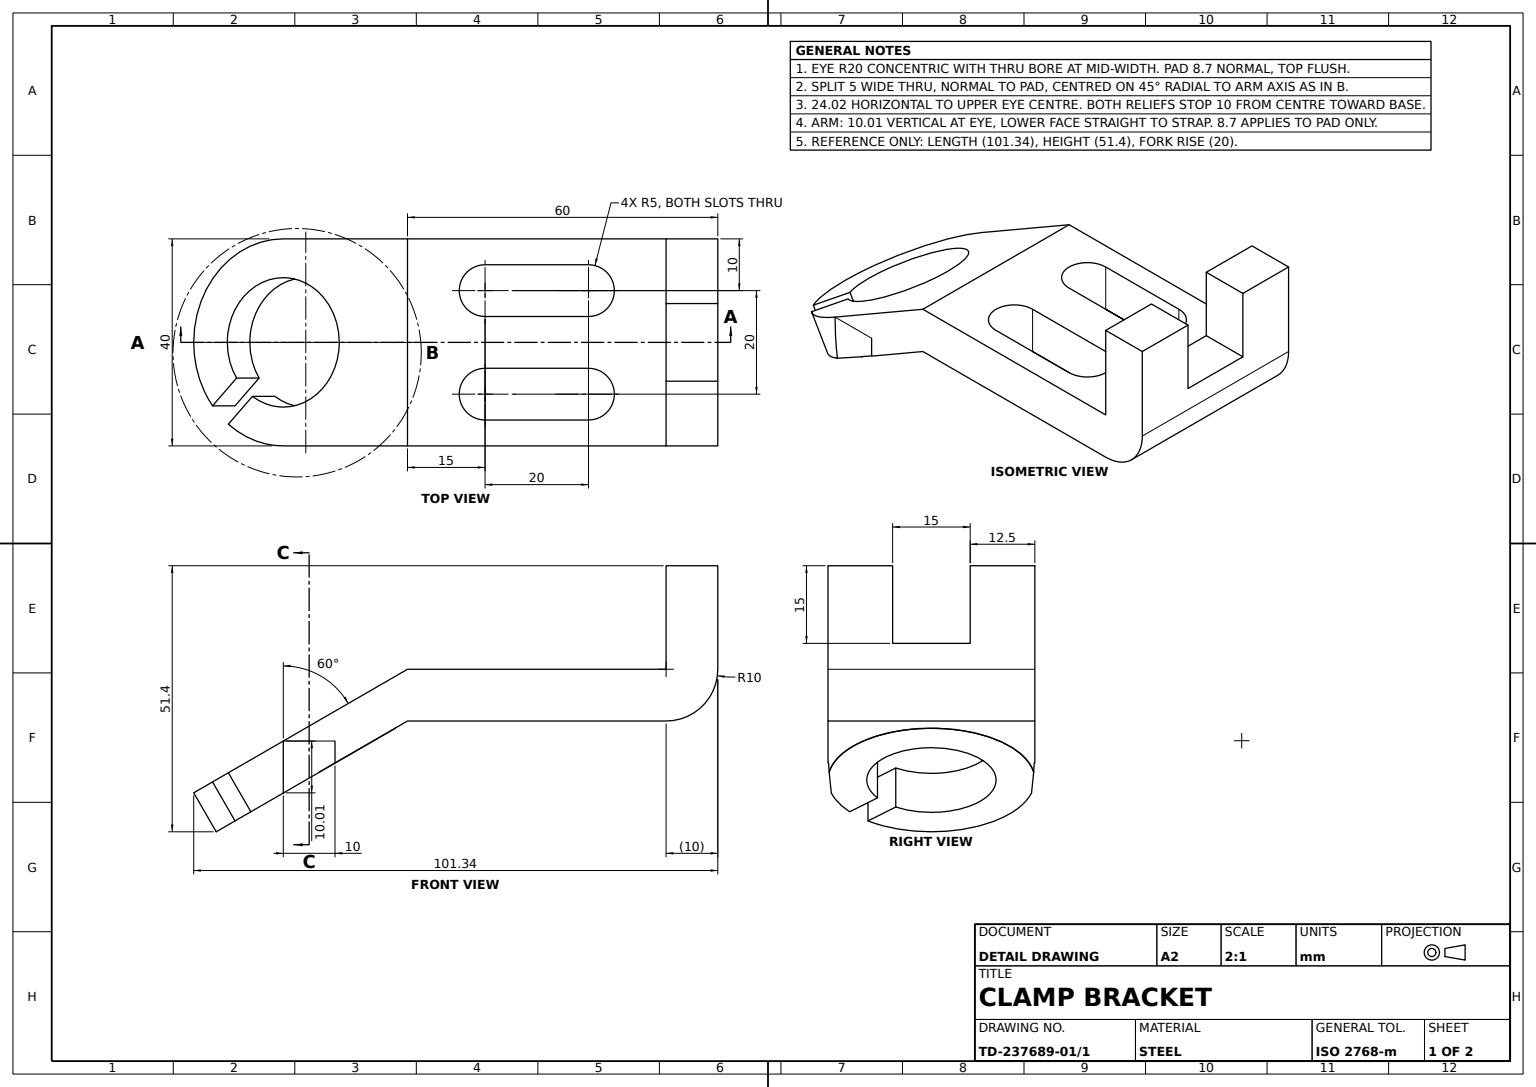
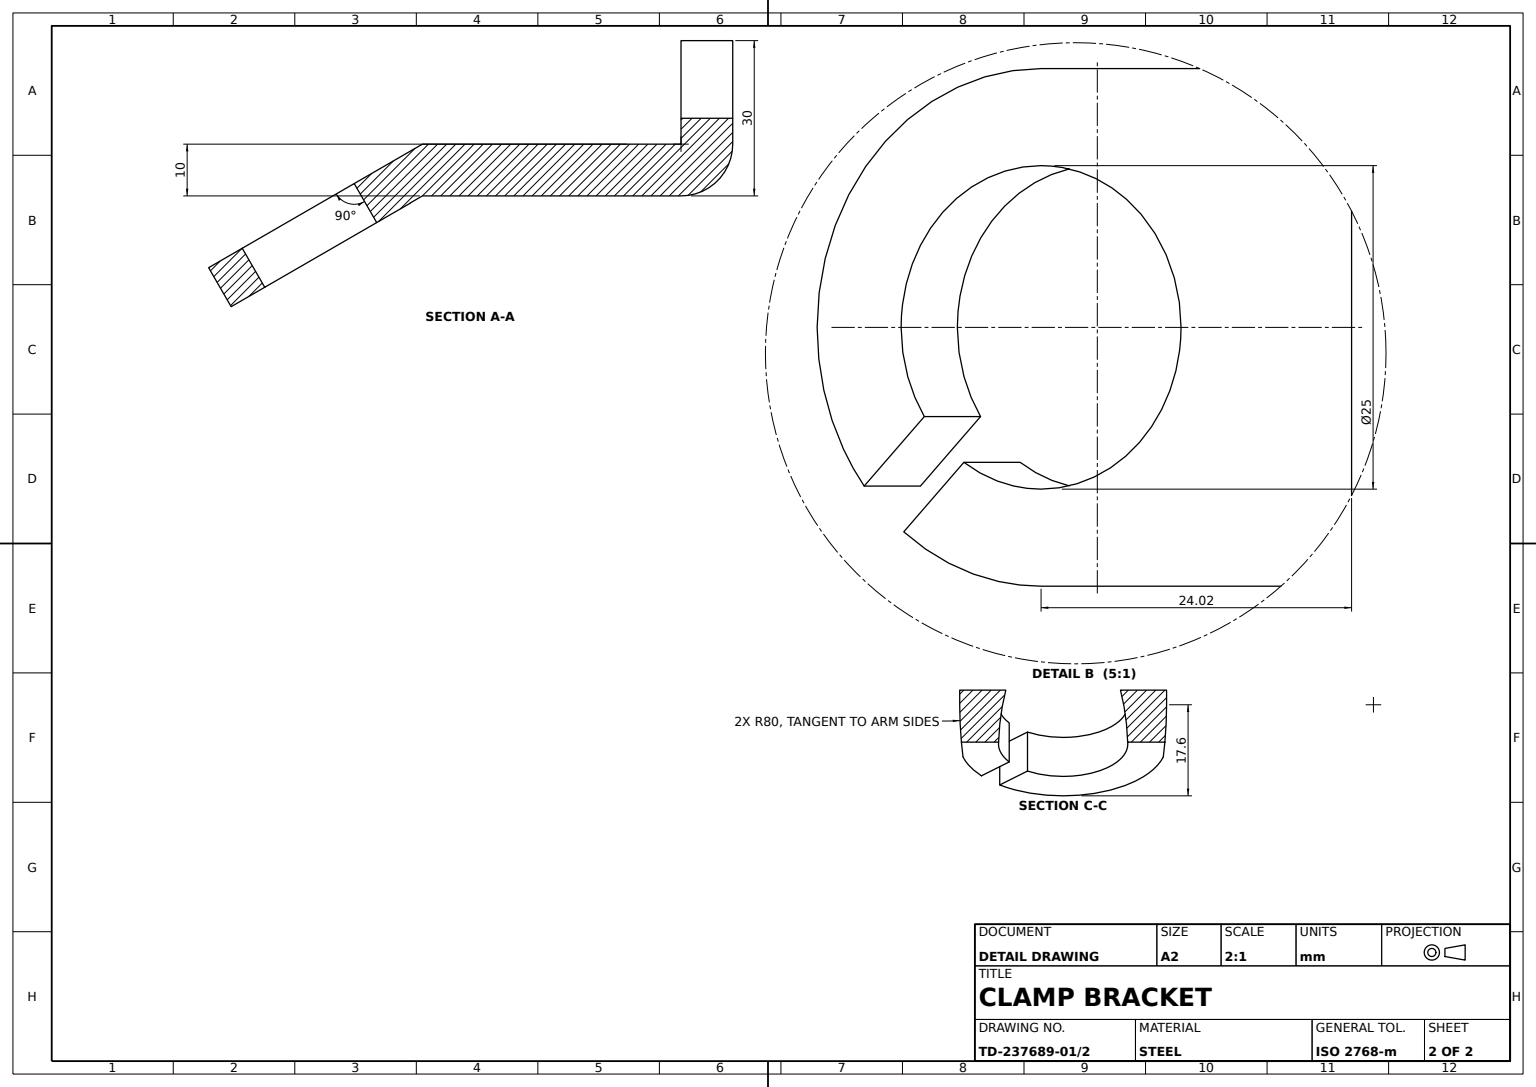
from build123d import *

# Parameters (mm, degrees)
L_BRACKET_BASE_DEPTH  = 40
CORNER_NOTCH_SKETCH_W = 15
CORNER_NOTCH_SKETCH_H = 15
CORNER_NOTCH_DEPTH    = 40
ANGLED_EYE_ARM_DEPTH  = 40
EYE_PAD_SKETCH_R      = 20
EYE_PAD_DEPTH         = 8.7
SLOT_1_DEPTH          = 10
SLOT_2_DEPTH          = 10
SPLIT_EYE_CUT_DEPTH   = 10
U_FORK_CUT_DEPTH      = 10


with BuildPart() as part:
    # L-Profile Sketch → L-Bracket Base (new body)
    with BuildSketch(Plane.XY):
        with BuildLine():
            Line((0, 0), (50, 0))
            ThreePointArc((50, 0), (57.071067812, 2.928932188), (60, 10))
            Line((60, 10), (60, 30))
            Line((60, 30), (50, 30))
            Line((50, 30), (50, 10))
            Line((50, 10), (0, 10))
            Line((0, 10), (0, 0))
        make_face()
    extrude(amount=-L_BRACKET_BASE_DEPTH)

    # Corner Notch Sketch → Corner Notch (cut)
    with BuildSketch(Plane.ZY.offset(-50)):
        with Locations((-20, 22.5)):
            Rectangle(CORNER_NOTCH_SKETCH_W, CORNER_NOTCH_SKETCH_H)
    extrude(amount=-CORNER_NOTCH_DEPTH, mode=Mode.SUBTRACT)

    # Angled Arm Sketch 60deg → Angled Eye Arm (add)
    with BuildSketch(Plane.XY):
        Polygon((-24.016551345, -13.87470631), (-24.016551345, -3.865962384), (0, 10), (0, 0), align=None)
    extrude(amount=-ANGLED_EYE_ARM_DEPTH)

    # Eye Pad Sketch → Eye Pad (add)
    with BuildSketch(Plane(origin=(-4.330127019, 7.5, 0), x_dir=(0.8660254037844397, 0.4999999999999981, 0), z_dir=(-0.4999999999999982, 0.8660254037844398, 0))):
        with Locations(Location((-22.731924769, 20, 0), (0, 0, 180))):
            Circle(EYE_PAD_SKETCH_R)
    extrude(amount=-EYE_PAD_DEPTH)

    # Slot 1 Sketch → Slot 1 (cut)
    with BuildSketch(Plane.ZY.offset(24.016551345)):
        with BuildLine():
            Line((-0.636212631, -13.87470631), (0, -13.87470631))
            Line((0, -13.87470631), (0, -3.865962384))
            ThreePointArc((0, -3.865962384), (-0.161112689, -8.880313754), (-0.636212631, -13.87470631))
        make_face()
    extrude(amount=-SLOT_1_DEPTH, mode=Mode.SUBTRACT)

    # Slot 2 Sketch → Slot 2 (cut)
    with BuildSketch(Plane.ZY.offset(24.016551345)):
        with BuildLine():
            Line((-40, -13.87470631), (-40, -3.865962384))
            ThreePointArc((-40, -3.865962384), (-39.838887311, -8.880313754), (-39.363787369, -13.87470631))
            Line((-39.363787369, -13.87470631), (-40, -13.87470631))
        make_face()
    extrude(amount=-SLOT_2_DEPTH, mode=Mode.SUBTRACT)

    # Split Eye Sketch → Split Eye Cut (cut)
    with BuildSketch(Plane(origin=(-4.330127019, 7.5, 0), x_dir=(0.8660254037844397, 0.4999999999999981, 0), z_dir=(-0.4999999999999982, 0.8660254037844398, 0))):
        with BuildLine():
            Line((-38.530906922, 7.736551753), (-33.159945759, 13.107512915))
            ThreePointArc((-33.159945759, 13.107512915), (-13.893090004, 28.838834765), (-29.624411853, 9.571979009))
            Line((-29.624411853, 9.571979009), (-34.995373016, 4.201017847))
            ThreePointArc((-34.995373016, 4.201017847), (-36.874060392, 5.857864376), (-38.530906922, 7.736551753))
        make_face()
    extrude(amount=-SPLIT_EYE_CUT_DEPTH, mode=Mode.SUBTRACT)

    # U-Fork Sketch → U-Fork Cut (cut)
    with BuildSketch(Plane(origin=(0, 10, 0), x_dir=(1, 0, 0), z_dir=(0, 1, 0))):
        with BuildLine():
            Line((15, 25), (35, 25))
            ThreePointArc((35, 25), (40, 30), (35, 35))
            Line((35, 35), (15, 35))
            ThreePointArc((15, 35), (10, 30), (15, 25))
        make_face()
        with BuildLine():
            Line((15, 5), (35, 5))
            ThreePointArc((35, 5), (40, 10), (35, 15))
            Line((35, 15), (15, 15))
            ThreePointArc((15, 15), (10, 10), (15, 5))
        make_face()
    extrude(amount=-U_FORK_CUT_DEPTH, mode=Mode.SUBTRACT)


solid = part.part
